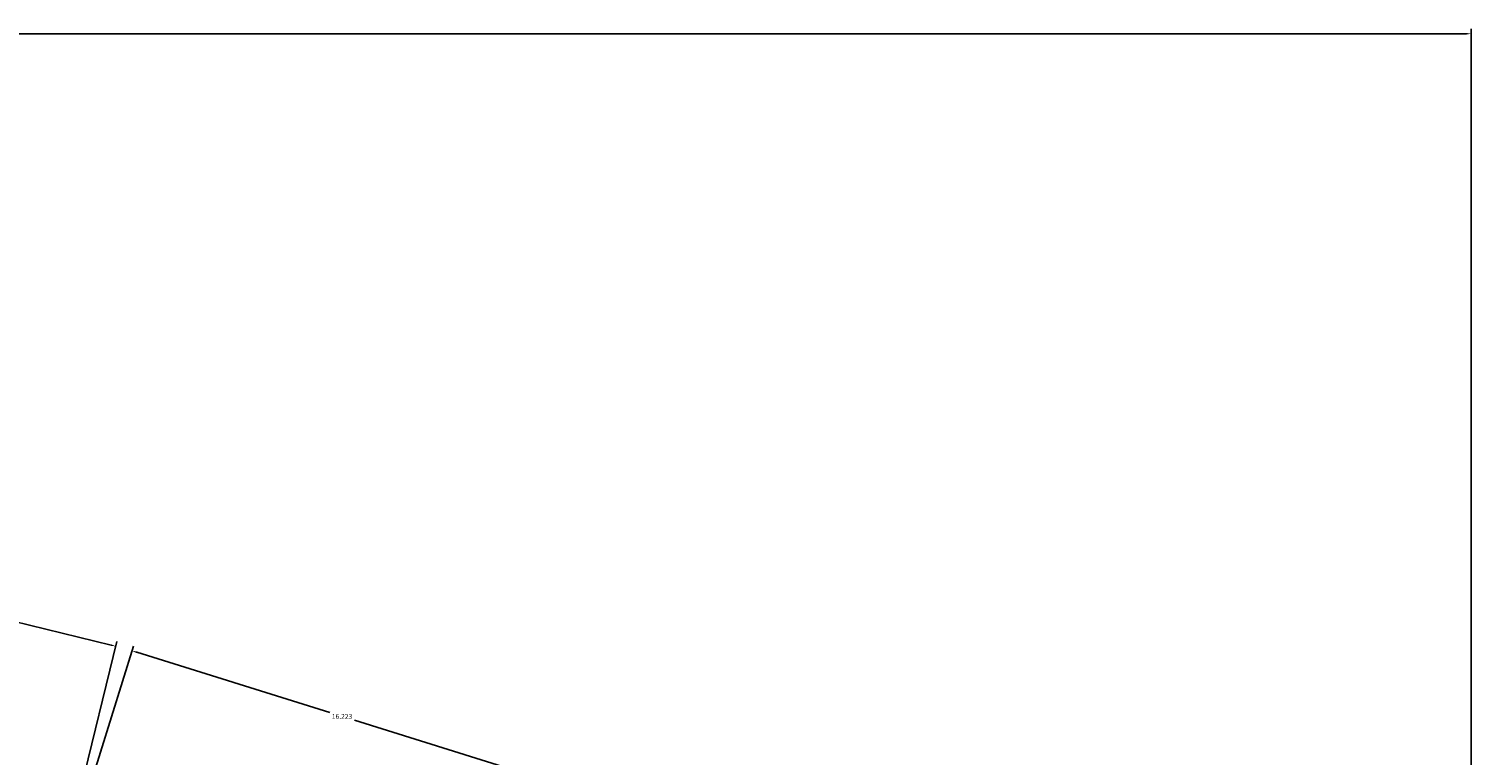
# Model space of a CAD drawing. Units: inches. Extents: x 413 to 622, y 326 to 447.
# Tile 15 of 15: x 568 to 622, y 420 to 447. Entities that reach past the tile are written whole.
import ezdxf

# ---------------------------------------------------------------- set-up
doc = ezdxf.new("R2010")
doc.units = ezdxf.units.IN
doc.header["$MEASUREMENT"] = 0
doc.layers.add('M-DIMS', color=2, linetype='Continuous', lineweight=18)
doc.styles.get("Standard").update_dxf_attribs({"font": 'arial.ttf'})
doc.dimstyles.get("Standard").update_dxf_attribs({"dimtxt": 0.18, "dimasz": 0.18, "dimexe": 0.18, "dimexo": 0.0625, "dimgap": 0.09, "dimtad": 0, "dimtih": 1, "dimtoh": 1, "dimdec": 4, "dimzin": 0, "dimdsep": 46, "dimtxsty": 'Standard', "dimcen": 0.09, "dimadec": 0, "dimazin": 0, "dimtfac": 1, "dimtdec": 4, "dimtofl": 0, "dimtmove": 0, "dimatfit": 3, "dimfxl": 1, "dimtolj": 1, "dimtzin": 0, "dimarcsym": 0})

# ---------------------------------------------------------------- blocks, each defined once
blk = doc.blocks.new('*D11')
at = {"layer": 'Defpoints', "color": 0, "transparency": 16777216}
for p in [(621.66, 446.422), (621.66, 388.074), (423.314, 378.888)]:
    blk.add_point(p, dxfattribs=at)
at = {"layer": 'M-DIMS', "color": 0, "lineweight": -2, "transparency": 16777216}
for p, q in [((423.314, 378.95), (423.314, 446.602)), ((621.66, 388.137), (621.66, 446.602)), ((423.494, 446.422), (522.031, 446.422)), ((621.48, 446.422), (522.943, 446.422))]:
    blk.add_line(p, q, dxfattribs=at)
at = {"layer": 'M-DIMS', "color": 0, "transparency": 16777216}
for points in [[(423.494, 446.452), (423.494, 446.392), (423.314, 446.422)], [(621.48, 446.452), (621.48, 446.392), (621.66, 446.422)]]:
    blk.add_solid(points, dxfattribs=at)
at = {"layer": 'M-DIMS', "color": 0, "transparency": 16777216, "insert": (522.487, 446.422), "char_height": 0.18, "attachment_point": 5}
blk.add_mtext('\\A1;198.35', dxfattribs=at)
blk = doc.blocks.new('*D21')
at = {"layer": 'Defpoints', "color": 0, "transparency": 16777216}
for p in [(571.652, 423.827), (549.452, 418.938), (569.266, 414.085)]:
    blk.add_point(p, dxfattribs=at)
at = {"layer": 'M-DIMS', "color": 0, "lineweight": -2, "transparency": 16777216}
for p, q in [((549.467, 418.998), (551.881, 428.855)), ((552.013, 428.637), (561.421, 426.333)), ((571.478, 423.87), (562.07, 426.174)), ((569.281, 414.145), (571.695, 424.002))]:
    blk.add_line(p, q, dxfattribs=at)
at = {"layer": 'M-DIMS', "color": 0, "transparency": 16777216}
for points in [[(552.02, 428.666), (552.006, 428.608), (551.838, 428.68)], [(571.485, 423.899), (571.47, 423.841), (571.652, 423.827)]]:
    blk.add_solid(points, dxfattribs=at)
at = {"layer": 'M-DIMS', "color": 0, "transparency": 16777216, "insert": (561.745, 426.254), "char_height": 0.18, "attachment_point": 5}
blk.add_mtext('\\A1;20.4', dxfattribs=at)
blk = doc.blocks.new('*D22')
at = {"layer": 'Defpoints', "color": 0, "transparency": 16777216}
for p in [(587.742, 418.825), (569.266, 414.085), (584.753, 409.25)]:
    blk.add_point(p, dxfattribs=at)
at = {"layer": 'M-DIMS', "color": 0, "lineweight": -2, "transparency": 16777216}
for p, q in [((569.285, 414.144), (572.309, 423.831)), ((572.427, 423.606), (579.543, 421.384)), ((587.57, 418.879), (580.454, 421.1)), ((584.771, 409.31), (587.795, 418.997))]:
    blk.add_line(p, q, dxfattribs=at)
at = {"layer": 'M-DIMS', "color": 0, "transparency": 16777216}
for points in [[(572.436, 423.635), (572.418, 423.577), (572.255, 423.66)], [(587.579, 418.907), (587.561, 418.85), (587.742, 418.825)]]:
    blk.add_solid(points, dxfattribs=at)
at = {"layer": 'M-DIMS', "color": 0, "transparency": 16777216, "insert": (579.999, 421.242), "char_height": 0.18, "attachment_point": 5}
blk.add_mtext('\\A1;16.223', dxfattribs=at)

msp = doc.modelspace()

# ---------------------------------------------------------------- dimensions: what is measured, and where the dimension line sits
at = {"layer": 'M-DIMS'}
dim = msp.add_linear_dim(base=(621.66, 446.422), p1=(423.3136, 378.8878), p2=(621.66, 388.0741), dimstyle='Standard', override={"dimdec": 2, "dimlfac": 1, "dimrnd": 0, "dimzin": 0, "dimdsep": 46, "dimlunit": 2}, dxfattribs=at)
dim.commit()
dim.dimension.update_dxf_attribs({"geometry": '*D11', "text_midpoint": (522.4868, 446.422)})
for base, p1, p2, angle, override, picture, middle in [((571.6524, 423.8274), (549.4524, 418.9375), (569.2663, 414.0848), 346.23831, {"dimdec": 1, "dimlfac": 1, "dimrnd": 0, "dimzin": 0, "dimdsep": 46, "dimlunit": 2}, '*D21', (561.7455, 426.2537)), ((587.7417, 418.8252), (569.2663, 414.0848), (584.7527, 409.2504), 342.66312, {"dimdec": 3, "dimlfac": 1, "dimrnd": 0, "dimzin": 0, "dimdsep": 46, "dimlunit": 2}, '*D22', (579.9985, 421.2424))]:
    dim = msp.add_linear_dim(base=base, p1=p1, p2=p2, angle=angle, dimstyle='Standard', override=override, dxfattribs=at)
    dim.commit()
    dim.dimension.update_dxf_attribs({"geometry": picture, "text_midpoint": middle})

doc.saveas('drawing.dxf')
